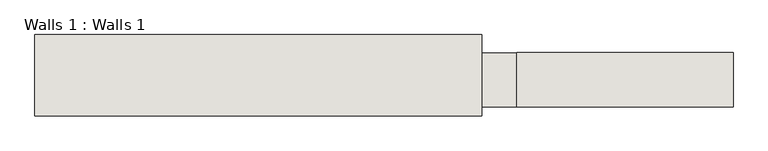
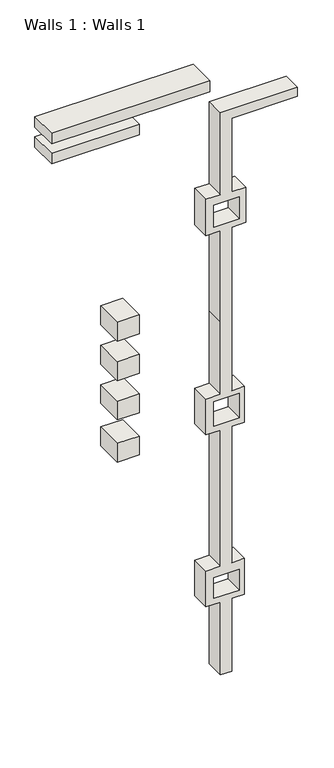
"""IFC4 building model written with IfcOpenShell, lengths in millimetres: wall geometry, Walls 1 : Walls 1."""

from ifc_helpers import new_model, si_unit, frame, origin, place, context, project, spatial, polyline, outline, extrude, source, transform, mapped, element, save


def walls_1_walls_1_5a20c518(model_context):
    return source(origin(), model_context, "Body", "SweptSolid", [
        extrude(outline(polyline([(10167.7423197, -2392.9093643), (8796.1423197, -2392.9093643), (8796.1423197, -2625.6369412), (8186.5423197, -2625.6369412), (8186.5423197, -2392.9093643), (6662.5423197, -2392.9093643), (5443.3423197, -2392.9093643), (5443.3423197, -2625.6369412), (4840.4971978, -2625.6369412), (4840.4971978, -2392.9093643), (2554.4971978, -2392.9093643), (2554.4971978, -2625.6369412), (1952.9020147, -2625.6369412), (1952.9020147, -2392.9093643), (733.7020147, -2392.9093643), (733.7020147, -2215.1093643), (1952.9020147, -2215.1093643), (1952.9020147, -2016.0369412), (2554.4971978, -2016.0369412), (2554.4971978, -2215.1093643), (4840.4971978, -2215.1093643), (4840.4971978, -2016.0369412), (5443.3423197, -2016.0369412), (5443.3423197, -2215.1093643), (8186.5423197, -2215.1093643), (8186.5423197, -1987.7443103), (8777.7221034, -1987.7443103), (8777.7221034, -2215.1093643), (10015.3423197, -2215.1093643), (10015.3423197, -1173.7093643), (10167.7423197, -1173.7093643), (10167.7423197, -2392.9093643)]), holes=[polyline([(5352.1532586, -2091.4945378), (4945.7532586, -2091.4945378), (4945.7532586, -2497.8945378), (5352.1532586, -2497.8945378), (5352.1532586, -2091.4945378)]), polyline([(2399.7768211, -2091.4945378), (2050.600569, -2091.4945378), (2050.600569, -2497.8945378), (2399.7768211, -2497.8945378), (2399.7768211, -2091.4945378)]), polyline([(8653.4950878, -2091.4945378), (8284.553898, -2091.4945378), (8284.553898, -2497.8945378), (8653.4950878, -2497.8945378), (8653.4950878, -2091.4945378)])]), frame((0.0, 1505.9827135, 0.0), z_axis=(0.0, 1.0, 0.0), x_axis=(0.0, 0.0, 1.0)), (0.0, 0.0, 1.0), 304.8),
        extrude(outline(polyline([(-2589.3419764, 1455.1827135), (-5103.9419764, 1455.1827135), (-5103.9419764, 1912.3827135), (-2589.3419764, 1912.3827135), (-2589.3419764, 1455.1827135)])), frame((0.0, 0.0, 10624.9423197), z_axis=(0.0, 0.0, 1.0), x_axis=(1.0, 0.0, 0.0)), (0.0, 0.0, 1.0), 177.8),
        extrude(outline(polyline([(-3706.9419764, 1455.1827135), (-5103.9419764, 1455.1827135), (-5103.9419764, 1912.3827135), (-3706.9419764, 1912.3827135), (-3706.9419764, 1455.1827135)])), frame((0.0, 0.0, 10292.4122632), z_axis=(0.0, 0.0, 1.0), x_axis=(1.0, 0.0, 0.0)), (0.0, 0.0, 1.0), 177.8),
        extrude(outline(polyline([(-3706.9419764, 1455.1827135), (-4060.4901493, 1455.1827135), (-4060.4901493, 1912.3827135), (-3706.9419764, 1912.3827135), (-3706.9419764, 1455.1827135)])), frame((0.0, 0.0, 6947.8866102), z_axis=(0.0, 0.0, 1.0), x_axis=(1.0, 0.0, 0.0)), (0.0, 0.0, 1.0), 316.5133898),
        extrude(outline(polyline([(-3706.9419764, 1455.1827135), (-4060.4901493, 1455.1827135), (-4060.4901493, 1912.3827135), (-3706.9419764, 1912.3827135), (-3706.9419764, 1455.1827135)])), frame((0.0, 0.0, 6287.4866102), z_axis=(0.0, 0.0, 1.0), x_axis=(1.0, 0.0, 0.0)), (0.0, 0.0, 1.0), 316.5133898),
        extrude(outline(polyline([(-3706.9419764, 1455.1827135), (-4060.4901493, 1455.1827135), (-4060.4901493, 1912.3827135), (-3706.9419764, 1912.3827135), (-3706.9419764, 1455.1827135)])), frame((0.0, 0.0, 5627.0866102), z_axis=(0.0, 0.0, 1.0), x_axis=(1.0, 0.0, 0.0)), (0.0, 0.0, 1.0), 316.5133898),
        extrude(outline(polyline([(-3706.9419764, 1455.1827135), (-4060.4901493, 1455.1827135), (-4060.4901493, 1912.3827135), (-3706.9419764, 1912.3827135), (-3706.9419764, 1455.1827135)])), frame((0.0, 0.0, 4915.8866102), z_axis=(0.0, 0.0, 1.0), x_axis=(1.0, 0.0, 0.0)), (0.0, 0.0, 1.0), 316.5133898),
    ])


if __name__ == "__main__":
    model = new_model("IFC4")
    model_context = context("Model", 3, world=origin())
    ifc_project = project(units=[si_unit("LENGTHUNIT", "METRE", prefix="MILLI")], contexts=[model_context])
    site = spatial("IfcSite", under=ifc_project)
    building = spatial("IfcBuilding", under=site)
    placement = place(None, origin())
    walls_1_walls_1_shape = walls_1_walls_1_5a20c518(model_context)
    element("IfcWall", 1, ObjectType="Walls 1 : Walls 1", at=placement, inside=building, context=model_context, shape_type="MappedRepresentation", body=[
        mapped(walls_1_walls_1_shape, transform((0.0, 0.0, 0.0), x_axis=(1.0, 0.0, 0.0), y_axis=(0.0, 1.0, 0.0), z_axis=(0.0, 0.0, 1.0))),
    ])
    save(model, "model.ifc")

# Revit data of these elements
# Element 1 (IfcWall, "Walls 1 : Walls 1")
#   Materials on its faces: "Default Wall"
# Materials
#   "Default Wall": colour RGB 128 128 128, transparency 0
